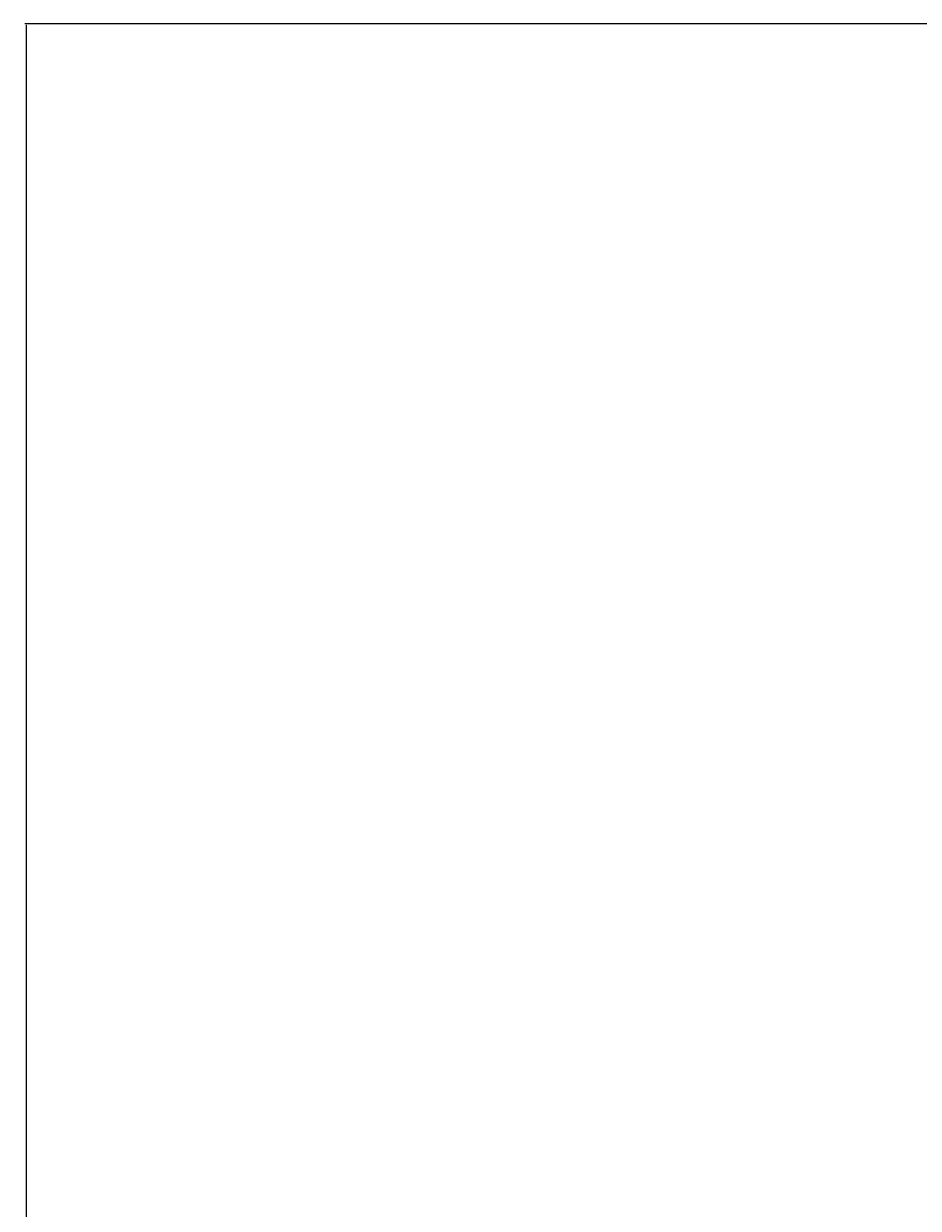
# Model space of a CAD drawing. Units: millimetres. Extents: x 27017497 to 27018854, y 7058029 to 7059154.
# Tile 43 of 91: x 27017497 to 27017611, y 7058472 to 7058623. Entities that reach past the tile are written whole.
import ezdxf

# ---------------------------------------------------------------- set-up
doc = ezdxf.new("R2010")
doc.units = ezdxf.units.MM
doc.layers.add('A-ANNO-DIMS', color=2, linetype='Continuous', lineweight=18)
doc.styles.get("Standard").update_dxf_attribs({"font": 'arial.ttf'})
doc.dimstyles.get("Standard").update_dxf_attribs({"dimtxt": 0.18, "dimasz": 0.18, "dimexe": 0.18, "dimexo": 0.0625, "dimgap": 0.09, "dimtad": 0, "dimtih": 1, "dimtoh": 1, "dimdec": 4, "dimzin": 0, "dimdsep": 46, "dimtxsty": 'Standard', "dimcen": 0.09, "dimadec": 0, "dimazin": 0, "dimtfac": 1, "dimtdec": 4, "dimtofl": 0, "dimtmove": 0, "dimatfit": 3, "dimfxl": 1, "dimtolj": 1, "dimtzin": 0, "dimarcsym": 0})

# ---------------------------------------------------------------- blocks, each defined once
blk = doc.blocks.new('*D48')
at = {"layer": 'A-ANNO-DIMS', "color": 0, "lineweight": -2, "transparency": 16777216}
for p, q in [((27018463.5, 7058622.91), (27017497.54, 7058622.91)), ((27017497.72, 7058622.73), (27017497.72, 7058357.75)), ((27017497.72, 7058092.41), (27017497.72, 7058357.39)), ((27018555.13, 7058092.23), (27017497.54, 7058092.23))]:
    blk.add_line(p, q, dxfattribs=at)
at = {"layer": 'A-ANNO-DIMS', "color": 0, "transparency": 16777216}
for points in [[(27017497.69, 7058622.73), (27017497.75, 7058622.73), (27017497.72, 7058622.91)], [(27017497.69, 7058092.41), (27017497.75, 7058092.41), (27017497.72, 7058092.23)]]:
    blk.add_solid(points, dxfattribs=at)
at = {"layer": 'Defpoints', "color": 0, "transparency": 16777216}
for p in [(27018463.56, 7058622.91), (27017497.72, 7058092.23), (27018555.19, 7058092.23)]:
    blk.add_point(p, dxfattribs=at)
at = {"layer": 'A-ANNO-DIMS', "color": 0, "transparency": 16777216, "insert": (27017497.72, 7058357.57), "char_height": 0.18, "attachment_point": 5}
blk.add_mtext('\\A1;530.7', dxfattribs=at)

msp = doc.modelspace()

# ---------------------------------------------------------------- dimensions: what is measured, and where the dimension line sits
at = {"layer": 'A-ANNO-DIMS'}
dim = msp.add_linear_dim(base=(27017497.716, 7058092.23), p1=(27018463.561, 7058622.912), p2=(27018555.192, 7058092.23), angle=90, dimstyle='Standard', override={"dimdec": 1, "dimlfac": 1, "dimrnd": 0, "dimzin": 0, "dimdsep": 46, "dimlunit": 2}, dxfattribs=at)
dim.commit()
dim.dimension.update_dxf_attribs({"geometry": '*D48', "text_midpoint": (27017497.716, 7058357.571)})

doc.saveas('drawing.dxf')
